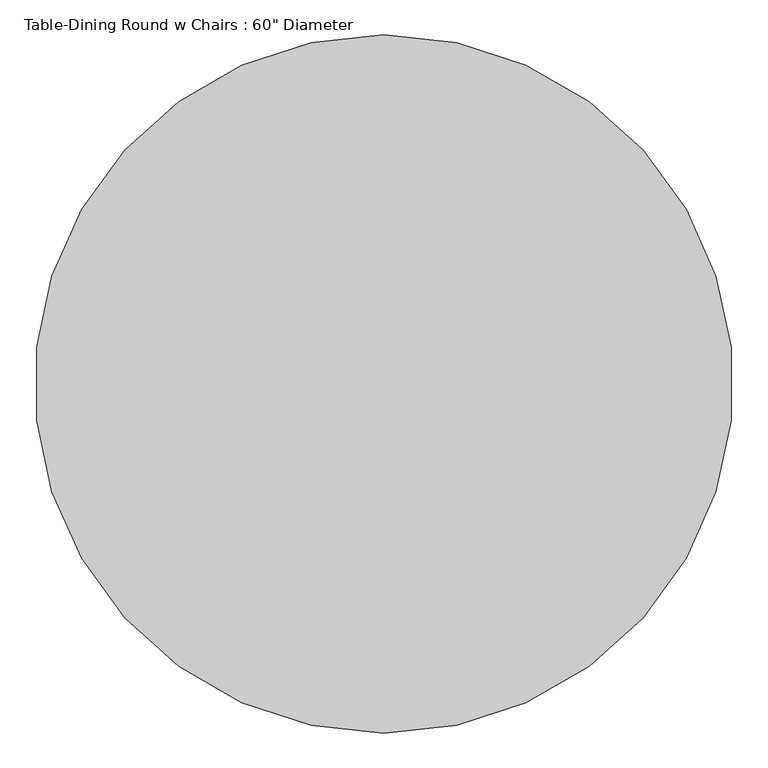
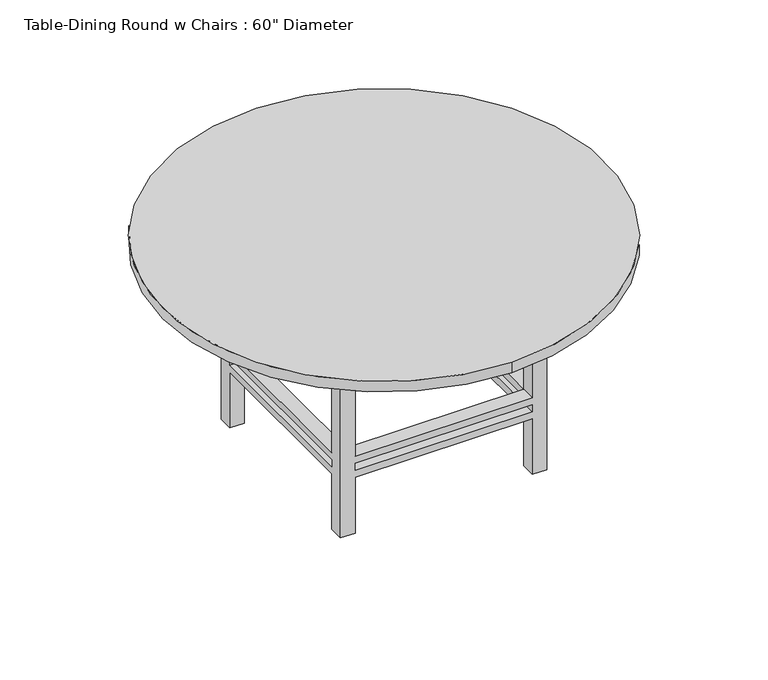
"""IFC4 building model written with IfcOpenShell, lengths in millimetres: furniture geometry."""

from ifc_helpers import new_model, si_unit, point, frame, frame_2d, origin, place, context, project, spatial, polyline, circle_curve, trimmed, segment, composite_curve, outline, extrude, faceted_brep, source, transform, mapped, element, save


def furniture_bbcc68ce(model_context):
    return source(origin(), model_context, "Body", "SolidModel", [
        faceted_brep([(408.4819672, 119.9213115, 279.4), (408.4819672, -489.6786885, 279.4), (459.2819672, -489.6786885, 279.4), (459.2819672, 119.9213115, 279.4), (-201.1180328, -489.6786885, 279.4), (-201.1180328, -540.4786885, 279.4), (408.4819672, -540.4786885, 279.4), (-201.1180328, 119.9213115, 279.4), (-251.9180328, 119.9213115, 279.4), (-251.9180328, -489.6786885, 279.4), (408.4819672, 170.7213115, 279.4), (-201.1180328, 170.7213115, 279.4), (408.4819672, 119.9213115, 254.0), (-201.1180328, 119.9213115, 254.0), (-201.1180328, 170.7213115, 254.0), (408.4819672, 170.7213115, 254.0), (-201.1180328, -489.6786885, 254.0), (-251.9180328, -489.6786885, 254.0), (-251.9180328, 119.9213115, 254.0), (408.4819672, -489.6786885, 254.0), (408.4819672, -540.4786885, 254.0), (-201.1180328, -540.4786885, 254.0), (459.2819672, 119.9213115, 254.0), (459.2819672, -489.6786885, 254.0), (-251.9180328, 170.7213115, 647.7), (-201.1180328, 170.7213115, 647.7), (408.4819672, 170.7213115, 647.7), (459.2819672, 170.7213115, 647.7), (459.2819672, 170.7213115, 0.0), (408.4819672, 170.7213115, 0.0), (408.4819672, 170.7213115, 203.2), (-201.1180328, 170.7213115, 203.2), (-201.1180328, 170.7213115, 0.0), (-251.9180328, 170.7213115, 0.0), (-201.1180328, 170.7213115, 228.6), (408.4819672, 170.7213115, 228.6), (-251.9180328, 119.9213115, 647.7), (-251.9180328, 119.9213115, 0.0), (-251.9180328, 119.9213115, 203.2), (-251.9180328, -489.6786885, 203.2), (-251.9180328, -489.6786885, 0.0), (-251.9180328, -540.4786885, 0.0), (-251.9180328, -540.4786885, 647.7), (-251.9180328, -489.6786885, 647.7), (-251.9180328, -489.6786885, 228.6), (-251.9180328, 119.9213115, 228.6), (459.2819672, -540.4786885, 647.7), (408.4819672, -540.4786885, 647.7), (-201.1180328, -540.4786885, 647.7), (-201.1180328, -540.4786885, 0.0), (-201.1180328, -540.4786885, 203.2), (408.4819672, -540.4786885, 203.2), (408.4819672, -540.4786885, 0.0), (459.2819672, -540.4786885, 0.0), (408.4819672, -540.4786885, 228.6), (-201.1180328, -540.4786885, 228.6), (459.2819672, 119.9213115, 647.7), (459.2819672, -489.6786885, 647.7), (459.2819672, -489.6786885, 0.0), (459.2819672, -489.6786885, 203.2), (459.2819672, 119.9213115, 203.2), (459.2819672, 119.9213115, 0.0), (459.2819672, 119.9213115, 228.6), (459.2819672, -489.6786885, 228.6), (-201.1180328, 119.9213115, 647.7), (408.4819672, -489.6786885, 647.7), (408.4819672, 119.9213115, 647.7), (-201.1180328, -489.6786885, 647.7), (408.4819672, 119.9213115, 0.0), (-201.1180328, -489.6786885, 0.0), (-201.1180328, 119.9213115, 0.0), (408.4819672, -489.6786885, 0.0), (-201.1180328, 119.9213115, 228.6), (-201.1180328, 119.9213115, 203.2), (408.4819672, 119.9213115, 228.6), (408.4819672, 119.9213115, 203.2), (408.4819672, -489.6786885, 228.6), (408.4819672, -489.6786885, 203.2), (-201.1180328, -489.6786885, 228.6), (-201.1180328, -489.6786885, 203.2)], [[[0, 1, 2, 3]], [[1, 4, 5, 6]], [[4, 7, 8, 9]], [[7, 0, 10, 11]], [[12, 13, 14, 15]], [[13, 16, 17, 18]], [[16, 19, 20, 21]], [[19, 12, 22, 23]], [[24, 25, 11, 10, 26, 27, 28, 29, 30, 31, 32, 33], [14, 34, 35, 15]], [[36, 24, 33, 37, 38, 39, 40, 41, 42, 43, 9, 8], [17, 44, 45, 18]], [[46, 47, 6, 5, 48, 42, 41, 49, 50, 51, 52, 53], [20, 54, 55, 21]], [[28, 27, 56, 3, 2, 57, 46, 53, 58, 59, 60, 61], [22, 62, 63, 23]], [[1, 0, 12, 19]], [[4, 1, 19, 16]], [[7, 4, 16, 13]], [[0, 7, 13, 12]], [[25, 24, 36, 64]], [[47, 46, 57, 65]], [[26, 66, 56, 27]], [[48, 67, 43, 42]], [[29, 28, 61, 68]], [[49, 41, 40, 69]], [[32, 70, 37, 33]], [[52, 71, 58, 53]], [[13, 18, 45, 72]], [[64, 36, 8, 7]], [[37, 70, 73, 38]], [[14, 13, 72, 34]], [[25, 64, 7, 11]], [[70, 32, 31, 73]], [[12, 15, 35, 74]], [[66, 26, 10, 0]], [[29, 68, 75, 30]], [[22, 12, 74, 62]], [[56, 66, 0, 3]], [[68, 61, 60, 75]], [[19, 23, 63, 76]], [[65, 57, 2, 1]], [[58, 71, 77, 59]], [[20, 19, 76, 54]], [[47, 65, 1, 6]], [[71, 52, 51, 77]], [[16, 21, 55, 78]], [[67, 48, 5, 4]], [[49, 69, 79, 50]], [[17, 16, 78, 44]], [[43, 67, 4, 9]], [[69, 40, 39, 79]], [[74, 76, 63, 62]], [[76, 78, 55, 54]], [[78, 72, 45, 44]], [[72, 74, 35, 34]], [[75, 73, 31, 30]], [[73, 79, 39, 38]], [[79, 77, 51, 50]], [[77, 75, 60, 59]], [[76, 74, 75, 77]], [[78, 76, 77, 79]], [[72, 78, 79, 73]], [[74, 72, 73, 75]]]),
        extrude(outline(polyline([(484.6819672, 196.1213115), (484.6819672, -565.8786885), (-277.3180328, -565.8786885), (-277.3180328, 196.1213115), (484.6819672, 196.1213115)]), holes=[polyline([(459.2819672, 170.7213115), (-251.9180328, 170.7213115), (-251.9180328, -540.4786885), (459.2819672, -540.4786885), (459.2819672, 170.7213115)])]), frame((0.0, 0.0, 647.7), z_axis=(0.0, 0.0, 1.0), x_axis=(1.0, 0.0, 0.0)), (0.0, 0.0, 1.0), 76.2),
        extrude(outline(composite_curve([segment(trimmed(circle_curve(frame_2d((103.6819672, -184.8786885)), 762.0), [point((103.6819672, -946.8786885))], [point((103.6819672, 577.1213115))], False, "CARTESIAN"), True, "CONTINUOUS"), segment(trimmed(circle_curve(frame_2d((103.6819672, -184.8786885)), 762.0), [point((103.6819672, 577.1213115))], [point((103.6819672, -946.8786885))], False, "CARTESIAN"), True, "CONTINUOUS")], self_intersect=False)), frame((0.0, 0.0, 723.9), z_axis=(0.0, 0.0, 1.0), x_axis=(1.0, 0.0, 0.0)), (0.0, 0.0, 1.0), 38.1),
    ])


if __name__ == "__main__":
    model = new_model("IFC4")
    model_context = context("Model", 3, world=origin())
    ifc_project = project(units=[si_unit("LENGTHUNIT", "METRE", prefix="MILLI")], contexts=[model_context])
    site = spatial("IfcSite", under=ifc_project)
    building = spatial("IfcBuilding", under=site)
    placement = place(None, origin())
    furniture_shape = furniture_bbcc68ce(model_context)
    element("IfcFurniture", 1, ObjectType="Table-Dining Round w Chairs : 60\" Diameter", at=placement, inside=building, context=model_context, shape_type="MappedRepresentation", body=[
        mapped(furniture_shape, transform((0.0, 0.0, 0.0), x_axis=(1.0, 0.0, 0.0), y_axis=(0.0, 1.0, 0.0), z_axis=(0.0, 0.0, 1.0))),
    ])
    save(model, "model.ifc")

# Revit data of these elements
# Type "Table-Dining Round w Chairs : 60\" Diameter"
#   Assembly Code = "E2020200"
#   Radius = 2' - 6"
#   Diameter = 5' - 0"
#   Height = 2' - 6"
#   Chairs = 6
#   Base Material = Pine
#   Top Material = Wood - Teak
#   Default Elevation = 0
# Element 1 (IfcFurniture, "Table-Dining Round w Chairs : 60\" Diameter")
#   Materials on its faces: "Pine", "Wood - Teak"
# Materials
#   "Pine": class "Wood", colour RGB 223 192 134, transparency 0, Description = "Pinus Echinata", Cost = 0
#   "Wood - Teak": class "Wood", colour RGB 145 112 90, transparency 0
